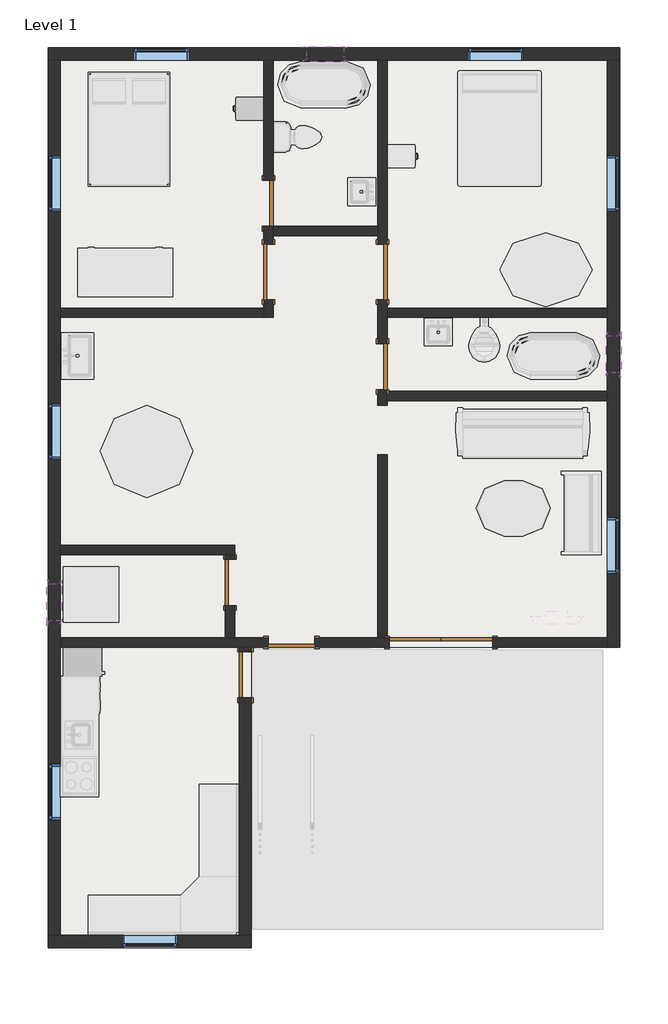
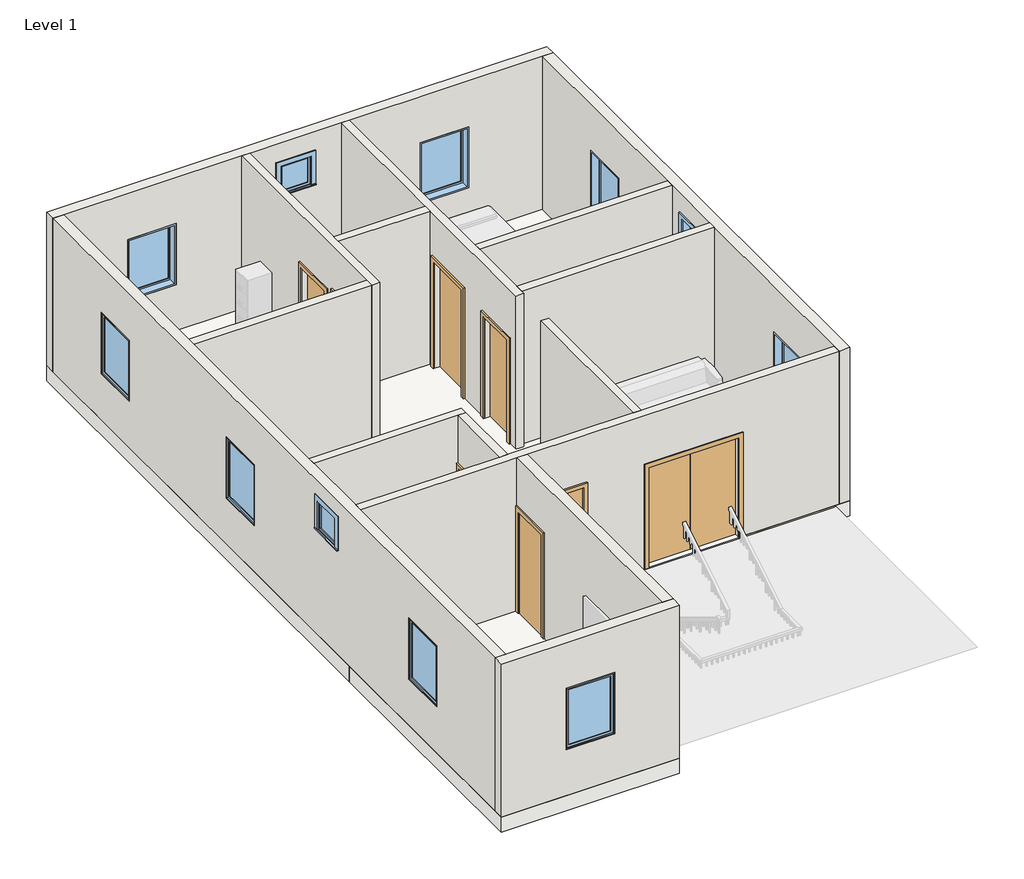
# One storey, part 1 of 3: 15 walls, 11 windows, 8 doors, 2 slabs.
"""IFC4 building model written with IfcOpenShell, lengths in millimetres."""

from ifc_helpers import new_model, si_unit, frame, origin, origin_with_axes, place, context, project, spatial, polyline, outline, extrude, faceted_brep, transform, mapped, element, save
from components import m_door_double_flush_panel_1700_x_2000mm_b668bbd0, door_059fdd7e, door_fadea3f2, door_686f89d2, door_16372e1c, window_e2841890, window_e41d21a6

model = new_model("IFC4")

# Units and contexts
model_context = context("Model", 3, world=origin())
ifc_project = project(units=[si_unit("LENGTHUNIT", "METRE", prefix="MILLI")], contexts=[model_context])

# Site, building, storey
site = spatial("IfcSite", under=ifc_project)
building = spatial("IfcBuilding", under=site)
storey = spatial("IfcBuildingStorey", under=building, Name="Level 1", Elevation=0.0)

# Doors
placement = place(None, origin())
m_door_double_flush_panel_1700_x_2000mm_shape = m_door_double_flush_panel_1700_x_2000mm_b668bbd0(model_context)
element("IfcDoor", 1, ObjectType="M_Door-Double-Flush_Panel : 1700 x 2000mm", at=placement, inside=storey, context=model_context, shape_type="MappedRepresentation", body=[
    mapped(m_door_double_flush_panel_1700_x_2000mm_shape, transform((-6764.5499219, 1169.9226537, 0.0), x_axis=(1.0, 0.0, 0.0), y_axis=(0.0, 1.0, 0.0), z_axis=(0.0, 0.0, 1.0))),
])
door_shape = door_059fdd7e(model_context)
element("IfcDoor", 2, ObjectType="Single-Flush : 30\" x 80\"", at=placement, inside=storey, context=model_context, shape_type="MappedRepresentation", body=[
    mapped(door_shape, transform((-9609.3499219, 8408.9226537, 0.0), x_axis=(0.0, -1.0, 0.0), y_axis=(1.0, 0.0, 0.0), z_axis=(0.0, 0.0, 1.0))),
])
element("IfcDoor", 3, ObjectType="Single-Flush : 30\" x 80\"", at=placement, inside=storey, context=model_context, shape_type="MappedRepresentation", body=[
    mapped(door_shape, transform((-7729.7499219, 5716.5226537, 0.0), x_axis=(0.0, -1.0, 0.0), y_axis=(1.0, 0.0, 0.0), z_axis=(0.0, 0.0, 1.0))),
])
element("IfcDoor", 4, ObjectType="Single-Flush : 30\" x 80\"", at=placement, inside=storey, context=model_context, shape_type="MappedRepresentation", body=[
    mapped(door_shape, transform((-10244.3499219, 2160.5226537, 0.0), x_axis=(0.0, 1.0, 0.0), y_axis=(-1.0, 0.0, 0.0), z_axis=(0.0, 0.0, 1.0))),
])
element("IfcDoor", 5, ObjectType="Single-Flush : 30\" x 80\"", at=placement, inside=storey, context=model_context, shape_type="MappedRepresentation", body=[
    mapped(door_shape, transform((-9228.3499219, 1169.9226537, 0.0), x_axis=(-1.0, 0.0, 0.0), y_axis=(0.0, -1.0, 0.0), z_axis=(0.0, 0.0, 1.0))),
])
door_2_shape = door_fadea3f2(model_context)
element("IfcDoor", 6, ObjectType="Single-Flush : 30\" x 80\"", at=placement, inside=storey, context=model_context, shape_type="MappedRepresentation", body=[
    mapped(door_2_shape, transform((-9990.3499219, 636.5226537, 0.0), x_axis=(0.0, 1.0, 0.0), y_axis=(-1.0, 0.0, 0.0), z_axis=(0.0, 0.0, 1.0))),
])
door_3_shape = door_686f89d2(model_context)
element("IfcDoor", 7, ObjectType="Single-Flush : 36\" x 84\"", at=placement, inside=storey, context=model_context, shape_type="MappedRepresentation", body=[
    mapped(door_3_shape, transform((-9609.3499219, 7278.6226537, 0.0), x_axis=(0.0, -1.0, 0.0), y_axis=(1.0, 0.0, 0.0), z_axis=(0.0, 0.0, 1.0))),
])
door_4_shape = door_16372e1c(model_context)
element("IfcDoor", 8, ObjectType="Single-Flush : 36\" x 84\"", at=placement, inside=storey, context=model_context, shape_type="MappedRepresentation", body=[
    mapped(door_4_shape, transform((-7729.7499219, 7278.6226537, 0.0), x_axis=(0.0, -1.0, 0.0), y_axis=(1.0, 0.0, 0.0), z_axis=(0.0, 0.0, 1.0))),
])

# Slabs
element("IfcSlab", 9, ObjectType="Generic - 12\"", at=placement, inside=storey, context=model_context, shape_type="SweptSolid", body=[
    extrude(outline(polyline([(-3818.1499219, 10974.3226537), (-3818.1499219, 1093.7226537), (-13241.5499219, 1093.7226537), (-13241.5499219, 10974.3226537), (-3818.1499219, 10974.3226537)])), frame((0.0, 0.0, -304.8), z_axis=(0.0, 0.0, 1.0), x_axis=(1.0, 0.0, 0.0)), (0.0, 0.0, 1.0), 304.8),
])
element("IfcSlab", 10, ObjectType="Generic - 12\"", at=placement, inside=storey, context=model_context, shape_type="SweptSolid", body=[
    extrude(outline(polyline([(-9888.7499219, 1093.7226537), (-9888.7499219, -3859.2773463), (-13241.5499219, -3859.2773463), (-13241.5499219, 1093.7226537), (-9888.7499219, 1093.7226537)])), frame((0.0, 0.0, -304.8), z_axis=(0.0, 0.0, 1.0), x_axis=(1.0, 0.0, 0.0)), (0.0, 0.0, 1.0), 304.8),
])

# Walls
element("IfcWall", 11, ObjectType="Generic - 8\"", at=placement, inside=storey, context=model_context, shape_type="Brep", body=[
    faceted_brep([(-13241.5499219, 10771.1226537, 0.0), (-13038.3499219, 10771.1226537, 0.0), (-9685.5499219, 10771.1226537, 0.0), (-9533.1499219, 10771.1226537, 0.0), (-7805.9499219, 10771.1226537, 0.0), (-7653.5499219, 10771.1226537, 0.0), (-4021.3499219, 10771.1226537, 0.0), (-3818.1499219, 10771.1226537, 0.0), (-3818.1499219, 10771.1226537, 3048.0), (-4021.3499219, 10771.1226537, 3048.0), (-7653.5499219, 10771.1226537, 3048.0), (-7805.9499219, 10771.1226537, 3048.0), (-9533.1499219, 10771.1226537, 3048.0), (-9685.5499219, 10771.1226537, 3048.0), (-13038.3499219, 10771.1226537, 3048.0), (-13241.5499219, 10771.1226537, 3048.0), (-10917.4499219, 10771.1226537, 2133.6), (-10917.4499219, 10771.1226537, 914.4), (-11831.8499219, 10771.1226537, 914.4), (-11831.8499219, 10771.1226537, 2133.6), (-5405.6499219, 10771.1226537, 2133.6), (-5405.6499219, 10771.1226537, 914.4), (-6320.0499219, 10771.1226537, 914.4), (-6320.0499219, 10771.1226537, 2133.6), (-8974.3499219, 10771.1226537, 2616.2), (-8364.7499219, 10771.1226537, 2616.2), (-8364.7499219, 10771.1226537, 2006.6), (-8974.3499219, 10771.1226537, 2006.6), (-13241.5499219, 10974.3226537, 0.0), (-13241.5499219, 10974.3226537, 3048.0), (-3818.1499219, 10974.3226537, 3048.0), (-3818.1499219, 10974.3226537, 0.0), (-10917.4499219, 10974.3226537, 2133.6), (-11831.8499219, 10974.3226537, 2133.6), (-11831.8499219, 10974.3226537, 914.4), (-10917.4499219, 10974.3226537, 914.4), (-5405.6499219, 10974.3226537, 2133.6), (-6320.0499219, 10974.3226537, 2133.6), (-6320.0499219, 10974.3226537, 914.4), (-5405.6499219, 10974.3226537, 914.4), (-8974.3499219, 10974.3226537, 2616.2), (-8974.3499219, 10974.3226537, 2006.6), (-8364.7499219, 10974.3226537, 2006.6), (-8364.7499219, 10974.3226537, 2616.2)], [[[0, 1, 2, 3, 4, 5, 6, 7, 8, 9, 10, 11, 12, 13, 14, 15], [16, 17, 18, 19], [20, 21, 22, 23], [24, 25, 26, 27]], [[28, 29, 30, 31], [32, 33, 34, 35], [36, 37, 38, 39], [40, 41, 42, 43]], [[7, 6, 5, 4, 3, 2, 1, 0, 28, 31]], [[15, 14, 13, 12, 11, 10, 9, 8, 30, 29]], [[8, 7, 31, 30]], [[0, 15, 29, 28]], [[17, 16, 32, 35]], [[18, 17, 35, 34]], [[19, 18, 34, 33]], [[16, 19, 33, 32]], [[21, 20, 36, 39]], [[22, 21, 39, 38]], [[23, 22, 38, 37]], [[20, 23, 37, 36]], [[41, 40, 24, 27]], [[42, 41, 27, 26]], [[43, 42, 26, 25]], [[40, 43, 25, 24]]]),
])
element("IfcWall", 12, ObjectType="Generic - 8\"", at=placement, inside=storey, context=model_context, shape_type="Brep", body=[
    faceted_brep([(-4021.3499219, 10771.1226537, 0.0), (-4021.3499219, 6681.7226537, 0.0), (-4021.3499219, 6529.3226537, 0.0), (-4021.3499219, 5310.1226537, 0.0), (-4021.3499219, 5157.7226537, 0.0), (-4021.3499219, 1246.1226537, 0.0), (-4021.3499219, 1093.7226537, 0.0), (-4021.3499219, 1093.7226537, 3048.0), (-4021.3499219, 1246.1226537, 3048.0), (-4021.3499219, 5157.7226537, 3048.0), (-4021.3499219, 5310.1226537, 3048.0), (-4021.3499219, 6529.3226537, 3048.0), (-4021.3499219, 6681.7226537, 3048.0), (-4021.3499219, 10771.1226537, 3048.0), (-4021.3499219, 8281.9226537, 2133.6), (-4021.3499219, 8281.9226537, 914.4), (-4021.3499219, 9196.3226537, 914.4), (-4021.3499219, 9196.3226537, 2133.6), (-4021.3499219, 2312.9226537, 2133.6), (-4021.3499219, 2312.9226537, 914.4), (-4021.3499219, 3227.3226537, 914.4), (-4021.3499219, 3227.3226537, 2133.6), (-4021.3499219, 5614.9226537, 2616.2), (-4021.3499219, 5614.9226537, 2006.6), (-4021.3499219, 6224.5226537, 2006.6), (-4021.3499219, 6224.5226537, 2616.2), (-3818.1499219, 10771.1226537, 0.0), (-3818.1499219, 10771.1226537, 3048.0), (-3818.1499219, 1093.7226537, 3048.0), (-3818.1499219, 1093.7226537, 0.0), (-3818.1499219, 8281.9226537, 2133.6), (-3818.1499219, 9196.3226537, 2133.6), (-3818.1499219, 9196.3226537, 914.4), (-3818.1499219, 8281.9226537, 914.4), (-3818.1499219, 2312.9226537, 2133.6), (-3818.1499219, 3227.3226537, 2133.6), (-3818.1499219, 3227.3226537, 914.4), (-3818.1499219, 2312.9226537, 914.4), (-3818.1499219, 5614.9226537, 2616.2), (-3818.1499219, 6224.5226537, 2616.2), (-3818.1499219, 6224.5226537, 2006.6), (-3818.1499219, 5614.9226537, 2006.6)], [[[0, 1, 2, 3, 4, 5, 6, 7, 8, 9, 10, 11, 12, 13], [14, 15, 16, 17], [18, 19, 20, 21], [22, 23, 24, 25]], [[26, 27, 28, 29], [30, 31, 32, 33], [34, 35, 36, 37], [38, 39, 40, 41]], [[6, 5, 4, 3, 2, 1, 0, 26, 29]], [[13, 12, 11, 10, 9, 8, 7, 28, 27]], [[0, 13, 27, 26]], [[7, 6, 29, 28]], [[15, 14, 30, 33]], [[16, 15, 33, 32]], [[17, 16, 32, 31]], [[14, 17, 31, 30]], [[19, 18, 34, 37]], [[20, 19, 37, 36]], [[21, 20, 36, 35]], [[18, 21, 35, 34]], [[23, 22, 38, 41]], [[24, 23, 41, 40]], [[25, 24, 40, 39]], [[22, 25, 39, 38]]]),
])
element("IfcWall", 13, ObjectType="Generic - 8\"", at=placement, inside=storey, context=model_context, shape_type="Brep", body=[
    faceted_brep([(-13038.3499219, -3656.0773463, 0.0), (-13038.3499219, 1093.7226537, 0.0), (-13038.3499219, 1246.1226537, 0.0), (-13038.3499219, 2617.7226537, 0.0), (-13038.3499219, 2770.1226537, 0.0), (-13038.3499219, 6529.3226537, 0.0), (-13038.3499219, 6681.7226537, 0.0), (-13038.3499219, 10771.1226537, 0.0), (-13038.3499219, 10771.1226537, 3048.0), (-13038.3499219, 6681.7226537, 3048.0), (-13038.3499219, 6529.3226537, 3048.0), (-13038.3499219, 2770.1226537, 3048.0), (-13038.3499219, 2617.7226537, 3048.0), (-13038.3499219, 1246.1226537, 3048.0), (-13038.3499219, 1093.7226537, 3048.0), (-13038.3499219, -3656.0773463, 3048.0), (-13038.3499219, -836.6773463, 2133.6), (-13038.3499219, -836.6773463, 914.4), (-13038.3499219, -1751.0773463, 914.4), (-13038.3499219, -1751.0773463, 2133.6), (-13038.3499219, 5106.9226537, 2133.6), (-13038.3499219, 5106.9226537, 914.4), (-13038.3499219, 4192.5226537, 914.4), (-13038.3499219, 4192.5226537, 2133.6), (-13038.3499219, 9196.3226537, 2133.6), (-13038.3499219, 9196.3226537, 914.4), (-13038.3499219, 8281.9226537, 914.4), (-13038.3499219, 8281.9226537, 2133.6), (-13038.3499219, 2135.1226537, 2692.4), (-13038.3499219, 2135.1226537, 2082.8), (-13038.3499219, 1525.5226537, 2082.8), (-13038.3499219, 1525.5226537, 2692.4), (-13241.5499219, -3656.0773463, 0.0), (-13241.5499219, -3656.0773463, 3048.0), (-13241.5499219, 10771.1226537, 3048.0), (-13241.5499219, 10771.1226537, 0.0), (-13241.5499219, -836.6773463, 2133.6), (-13241.5499219, -1751.0773463, 2133.6), (-13241.5499219, -1751.0773463, 914.4), (-13241.5499219, -836.6773463, 914.4), (-13241.5499219, 5106.9226537, 2133.6), (-13241.5499219, 4192.5226537, 2133.6), (-13241.5499219, 4192.5226537, 914.4), (-13241.5499219, 5106.9226537, 914.4), (-13241.5499219, 9196.3226537, 2133.6), (-13241.5499219, 8281.9226537, 2133.6), (-13241.5499219, 8281.9226537, 914.4), (-13241.5499219, 9196.3226537, 914.4), (-13241.5499219, 2135.1226537, 2692.4), (-13241.5499219, 1525.5226537, 2692.4), (-13241.5499219, 1525.5226537, 2082.8), (-13241.5499219, 2135.1226537, 2082.8)], [[[0, 1, 2, 3, 4, 5, 6, 7, 8, 9, 10, 11, 12, 13, 14, 15], [16, 17, 18, 19], [20, 21, 22, 23], [24, 25, 26, 27], [28, 29, 30, 31]], [[32, 33, 34, 35], [36, 37, 38, 39], [40, 41, 42, 43], [44, 45, 46, 47], [48, 49, 50, 51]], [[7, 6, 5, 4, 3, 2, 1, 0, 32, 35]], [[15, 14, 13, 12, 11, 10, 9, 8, 34, 33]], [[8, 7, 35, 34]], [[0, 15, 33, 32]], [[17, 16, 36, 39]], [[18, 17, 39, 38]], [[19, 18, 38, 37]], [[16, 19, 37, 36]], [[21, 20, 40, 43]], [[22, 21, 43, 42]], [[23, 22, 42, 41]], [[20, 23, 41, 40]], [[25, 24, 44, 47]], [[26, 25, 47, 46]], [[27, 26, 46, 45]], [[24, 27, 45, 44]], [[29, 28, 48, 51]], [[30, 29, 51, 50]], [[31, 30, 50, 49]], [[28, 31, 49, 48]]]),
])
element("IfcWall", 14, ObjectType="Generic - 8\"", at=placement, inside=storey, context=model_context, shape_type="SweptSolid", body=[
    extrude(outline(polyline([(1093.7226537, 0.0), (1017.5226537, 0.0), (1017.5226537, 2032.0), (255.5226537, 2032.0), (255.5226537, 0.0), (-3656.0773463, 0.0), (-3656.0773463, 3048.0), (1093.7226537, 3048.0), (1093.7226537, 0.0)])), frame((-10091.9499219, 0.0, 0.0), z_axis=(1.0, 0.0, 0.0), x_axis=(0.0, 1.0, 0.0)), (0.0, 0.0, 1.0), 203.2),
])
element("IfcWall", 15, ObjectType="Generic - 8\"", at=placement, inside=storey, context=model_context, shape_type="Brep", body=[
    faceted_brep([(-9888.7499219, -3656.0773463, 0.0), (-10091.9499219, -3656.0773463, 0.0), (-13038.3499219, -3656.0773463, 0.0), (-13241.5499219, -3656.0773463, 0.0), (-13241.5499219, -3656.0773463, 3048.0), (-13038.3499219, -3656.0773463, 3048.0), (-10091.9499219, -3656.0773463, 3048.0), (-9888.7499219, -3656.0773463, 3048.0), (-12022.3499219, -3656.0773463, 2133.6), (-12022.3499219, -3656.0773463, 914.4), (-11107.9499219, -3656.0773463, 914.4), (-11107.9499219, -3656.0773463, 2133.6), (-9888.7499219, -3859.2773463, 0.0), (-9888.7499219, -3859.2773463, 3048.0), (-13241.5499219, -3859.2773463, 3048.0), (-13241.5499219, -3859.2773463, 0.0), (-12022.3499219, -3859.2773463, 2133.6), (-11107.9499219, -3859.2773463, 2133.6), (-11107.9499219, -3859.2773463, 914.4), (-12022.3499219, -3859.2773463, 914.4)], [[[0, 1, 2, 3, 4, 5, 6, 7], [8, 9, 10, 11]], [[12, 13, 14, 15], [16, 17, 18, 19]], [[3, 2, 1, 0, 12, 15]], [[7, 6, 5, 4, 14, 13]], [[4, 3, 15, 14]], [[0, 7, 13, 12]], [[9, 8, 16, 19]], [[10, 9, 19, 18]], [[11, 10, 18, 17]], [[8, 11, 17, 16]]]),
])
element("IfcWall", 16, ObjectType="INNER WALL 6\"", at=placement, inside=storey, context=model_context, shape_type="Brep", body=[
    faceted_brep([(-9685.5499219, 8027.9226537, 2032.0), (-9685.5499219, 8027.9226537, 0.0), (-9685.5499219, 7735.8226537, 0.0), (-9685.5499219, 7735.8226537, 2133.6), (-9685.5499219, 6821.4226537, 2133.6), (-9685.5499219, 6821.4226537, 0.0), (-9685.5499219, 6681.7226537, 0.0), (-9685.5499219, 6529.3226537, 0.0), (-9685.5499219, 6529.3226537, 3048.0), (-9685.5499219, 6681.7226537, 3048.0), (-9685.5499219, 10771.1226537, 3048.0), (-9685.5499219, 10771.1226537, 0.0), (-9685.5499219, 8789.9226537, 0.0), (-9685.5499219, 8789.9226537, 2032.0), (-9533.1499219, 7735.8226537, 0.0), (-9533.1499219, 7875.5226537, 0.0), (-9533.1499219, 8027.9226537, 0.0), (-9533.1499219, 8027.9226537, 2032.0), (-9533.1499219, 8789.9226537, 2032.0), (-9533.1499219, 8789.9226537, 0.0), (-9533.1499219, 10771.1226537, 0.0), (-9533.1499219, 10771.1226537, 3048.0), (-9533.1499219, 8027.9226537, 3048.0), (-9533.1499219, 7875.5226537, 3048.0), (-9533.1499219, 6529.3226537, 3048.0), (-9533.1499219, 6529.3226537, 0.0), (-9533.1499219, 6821.4226537, 0.0), (-9533.1499219, 6821.4226537, 2133.6), (-9533.1499219, 7735.8226537, 2133.6)], [[[0, 1, 2, 3, 4, 5, 6, 7, 8, 9, 10, 11, 12, 13]], [[14, 15, 16, 17, 18, 19, 20, 21, 22, 23, 24, 25, 26, 27, 28]], [[7, 6, 5, 26, 25]], [[12, 11, 20, 19]], [[2, 1, 16, 15, 14]], [[10, 9, 8, 24, 23, 22, 21]], [[11, 10, 21, 20]], [[8, 7, 25, 24]], [[27, 26, 5, 4]], [[28, 27, 4, 3]], [[14, 28, 3, 2]], [[17, 16, 1, 0]], [[18, 17, 0, 13]], [[19, 18, 13, 12]]]),
])
element("IfcWall", 17, ObjectType="INNER WALL 6\"", at=placement, inside=storey, context=model_context, shape_type="SweptSolid", body=[
    extrude(outline(polyline([(-13038.3499219, 6681.7226537), (-9685.5499219, 6681.7226537), (-9685.5499219, 6529.3226537), (-13038.3499219, 6529.3226537), (-13038.3499219, 6681.7226537)])), origin_with_axes(), (0.0, 0.0, 1.0), 3048.0),
])
element("IfcWall", 18, ObjectType="INNER WALL 6\"", at=placement, inside=storey, context=model_context, shape_type="Brep", body=[
    faceted_brep([(-7805.9499219, 8027.9226537, 0.0), (-9533.1499219, 8027.9226537, 0.0), (-9533.1499219, 8027.9226537, 2032.0), (-9533.1499219, 8027.9226537, 3048.0), (-7805.9499219, 8027.9226537, 3048.0), (-7805.9499219, 7875.5226537, 0.0), (-7805.9499219, 7875.5226537, 3048.0), (-9533.1499219, 7875.5226537, 3048.0), (-9533.1499219, 7875.5226537, 0.0)], [[[0, 1, 2, 3, 4]], [[5, 6, 7, 8]], [[1, 0, 5, 8]], [[4, 3, 7, 6]], [[0, 4, 6, 5]], [[3, 2, 1, 8, 7]]]),
])
element("IfcWall", 19, ObjectType="INNER WALL 6\"", at=placement, inside=storey, context=model_context, shape_type="SweptSolid", body=[
    extrude(outline(polyline([(-4021.3499219, 6529.3226537), (-7653.5499219, 6529.3226537), (-7653.5499219, 6681.7226537), (-4021.3499219, 6681.7226537), (-4021.3499219, 6529.3226537)])), origin_with_axes(), (0.0, 0.0, 1.0), 3048.0),
])
element("IfcWall", 20, ObjectType="INNER WALL 6\"", at=placement, inside=storey, context=model_context, shape_type="Brep", body=[
    faceted_brep([(-13038.3499219, 2617.7226537, 0.0), (-10320.5499219, 2617.7226537, 0.0), (-10168.1499219, 2617.7226537, 0.0), (-10168.1499219, 2617.7226537, 3048.0), (-10320.5499219, 2617.7226537, 3048.0), (-13038.3499219, 2617.7226537, 3048.0), (-13038.3499219, 2770.1226537, 0.0), (-13038.3499219, 2770.1226537, 3048.0), (-10168.1499219, 2770.1226537, 3048.0), (-10168.1499219, 2770.1226537, 0.0)], [[[0, 1, 2, 3, 4, 5]], [[6, 7, 8, 9]], [[2, 1, 0, 6, 9]], [[5, 4, 3, 8, 7]], [[0, 5, 7, 6]], [[3, 2, 9, 8]]]),
])
element("IfcWall", 21, ObjectType="INNER WALL 6\"", at=placement, inside=storey, context=model_context, shape_type="Brep", body=[
    faceted_brep([(-4021.3499219, 1093.7226537, 3048.0), (-9888.7499219, 1093.7226537, 3048.0), (-10091.9499219, 1093.7226537, 3048.0), (-13038.3499219, 1093.7226537, 3048.0), (-13038.3499219, 1093.7226537, 0.0), (-10091.9499219, 1093.7226537, 0.0), (-9888.7499219, 1093.7226537, 0.0), (-9609.3499219, 1093.7226537, 0.0), (-9609.3499219, 1093.7226537, 2032.0), (-8847.3499219, 1093.7226537, 2032.0), (-8847.3499219, 1093.7226537, 0.0), (-7614.5499219, 1093.7226537, 0.0), (-7614.5499219, 1093.7226537, 2000.0), (-5914.5499219, 1093.7226537, 2000.0), (-5914.5499219, 1093.7226537, 0.0), (-4021.3499219, 1093.7226537, 0.0), (-13038.3499219, 1246.1226537, 3048.0), (-10320.5499219, 1246.1226537, 3048.0), (-10168.1499219, 1246.1226537, 3048.0), (-7805.9499219, 1246.1226537, 3048.0), (-7653.5499219, 1246.1226537, 3048.0), (-4021.3499219, 1246.1226537, 3048.0), (-4021.3499219, 1246.1226537, 0.0), (-5914.5499219, 1246.1226537, 0.0), (-5914.5499219, 1246.1226537, 2000.0), (-7614.5499219, 1246.1226537, 2000.0), (-7614.5499219, 1246.1226537, 0.0), (-7653.5499219, 1246.1226537, 0.0), (-7805.9499219, 1246.1226537, 0.0), (-8847.3499219, 1246.1226537, 0.0), (-8847.3499219, 1246.1226537, 2032.0), (-9609.3499219, 1246.1226537, 2032.0), (-9609.3499219, 1246.1226537, 0.0), (-10168.1499219, 1246.1226537, 0.0), (-10320.5499219, 1246.1226537, 0.0), (-13038.3499219, 1246.1226537, 0.0)], [[[0, 1, 2, 3, 4, 5, 6, 7, 8, 9, 10, 11, 12, 13, 14, 15]], [[16, 17, 18, 19, 20, 21, 22, 23, 24, 25, 26, 27, 28, 29, 30, 31, 32, 33, 34, 35]], [[4, 35, 34, 33, 32, 7, 6, 5]], [[22, 15, 14, 23]], [[10, 29, 28, 27, 26, 11]], [[3, 2, 1, 0, 21, 20, 19, 18, 17, 16]], [[4, 3, 16, 35]], [[0, 15, 22, 21]], [[8, 7, 32, 31]], [[9, 8, 31, 30]], [[10, 9, 30, 29]], [[13, 24, 23, 14]], [[24, 13, 12, 25]], [[25, 12, 11, 26]]]),
])
element("IfcWall", 22, ObjectType="INNER WALL 6\"", at=placement, inside=storey, context=model_context, shape_type="SweptSolid", body=[
    extrude(outline(polyline([(-7653.5499219, 4268.7226537), (-7653.5499219, 1246.1226537), (-7805.9499219, 1246.1226537), (-7805.9499219, 4268.7226537), (-7653.5499219, 4268.7226537)])), origin_with_axes(), (0.0, 0.0, 1.0), 3048.0),
])
element("IfcWall", 23, ObjectType="INNER WALL 6\"", at=placement, inside=storey, context=model_context, shape_type="SweptSolid", body=[
    extrude(outline(polyline([(-4021.3499219, 5157.7226537), (-7653.5499219, 5157.7226537), (-7653.5499219, 5310.1226537), (-4021.3499219, 5310.1226537), (-4021.3499219, 5157.7226537)])), origin_with_axes(), (0.0, 0.0, 1.0), 3048.0),
])
element("IfcWall", 24, ObjectType="INNER WALL 6\"", at=placement, inside=storey, context=model_context, shape_type="SweptSolid", body=[
    extrude(outline(polyline([(2617.7226537, 0.0), (2541.5226537, 0.0), (2541.5226537, 2032.0), (1779.5226537, 2032.0), (1779.5226537, 0.0), (1246.1226537, 0.0), (1246.1226537, 3048.0), (2617.7226537, 3048.0), (2617.7226537, 0.0)])), frame((-10320.5499219, 0.0, 0.0), z_axis=(1.0, 0.0, 0.0), x_axis=(0.0, 1.0, 0.0)), (0.0, 0.0, 1.0), 152.4),
])
element("IfcWall", 25, ObjectType="INNER WALL 6\"", at=placement, inside=storey, context=model_context, shape_type="Brep", body=[
    faceted_brep([(-7653.5499219, 5081.5226537, 0.0), (-7653.5499219, 5157.7226537, 0.0), (-7653.5499219, 5310.1226537, 0.0), (-7653.5499219, 5335.5226537, 0.0), (-7653.5499219, 5335.5226537, 2032.0), (-7653.5499219, 6097.5226537, 2032.0), (-7653.5499219, 6097.5226537, 0.0), (-7653.5499219, 6529.3226537, 0.0), (-7653.5499219, 6681.7226537, 0.0), (-7653.5499219, 6821.4226537, 0.0), (-7653.5499219, 6821.4226537, 2133.6), (-7653.5499219, 7735.8226537, 2133.6), (-7653.5499219, 7735.8226537, 0.0), (-7653.5499219, 10771.1226537, 0.0), (-7653.5499219, 10771.1226537, 3048.0), (-7653.5499219, 6681.7226537, 3048.0), (-7653.5499219, 6529.3226537, 3048.0), (-7653.5499219, 5310.1226537, 3048.0), (-7653.5499219, 5157.7226537, 3048.0), (-7653.5499219, 5081.5226537, 3048.0), (-7805.9499219, 5335.5226537, 2032.0), (-7805.9499219, 5335.5226537, 0.0), (-7805.9499219, 5081.5226537, 0.0), (-7805.9499219, 5081.5226537, 3048.0), (-7805.9499219, 7875.5226537, 3048.0), (-7805.9499219, 8027.9226537, 3048.0), (-7805.9499219, 10771.1226537, 3048.0), (-7805.9499219, 10771.1226537, 0.0), (-7805.9499219, 8027.9226537, 0.0), (-7805.9499219, 7875.5226537, 0.0), (-7805.9499219, 7735.8226537, 0.0), (-7805.9499219, 7735.8226537, 2133.6), (-7805.9499219, 6821.4226537, 2133.6), (-7805.9499219, 6821.4226537, 0.0), (-7805.9499219, 6097.5226537, 0.0), (-7805.9499219, 6097.5226537, 2032.0)], [[[0, 1, 2, 3, 4, 5, 6, 7, 8, 9, 10, 11, 12, 13, 14, 15, 16, 17, 18, 19]], [[20, 21, 22, 23, 24, 25, 26, 27, 28, 29, 30, 31, 32, 33, 34, 35]], [[34, 33, 9, 8, 7, 6]], [[22, 21, 3, 2, 1, 0]], [[30, 29, 28, 27, 13, 12]], [[19, 18, 17, 16, 15, 14, 26, 25, 24, 23]], [[0, 19, 23, 22]], [[14, 13, 27, 26]], [[12, 11, 31, 30]], [[11, 10, 32, 31]], [[10, 9, 33, 32]], [[6, 5, 35, 34]], [[5, 4, 20, 35]], [[4, 3, 21, 20]]]),
])

# Windows
window_shape = window_e2841890(model_context)
element("IfcWindow", 26, ObjectType="Fixed : 36\" x 48\"", at=placement, inside=storey, context=model_context, shape_type="MappedRepresentation", body=[
    mapped(window_shape, transform((-11603.2499219, -3757.6773463, 0.0), x_axis=(-1.0, 0.0, 0.0), y_axis=(0.0, -1.0, 0.0), z_axis=(0.0, 0.0, 1.0))),
])
element("IfcWindow", 27, ObjectType="Fixed : 36\" x 48\"", at=placement, inside=storey, context=model_context, shape_type="MappedRepresentation", body=[
    mapped(window_shape, transform((-13139.9499219, -1255.7773463, 0.0), x_axis=(0.0, 1.0, 0.0), y_axis=(-1.0, 0.0, 0.0), z_axis=(0.0, 0.0, 1.0))),
])
element("IfcWindow", 28, ObjectType="Fixed : 36\" x 48\"", at=placement, inside=storey, context=model_context, shape_type="MappedRepresentation", body=[
    mapped(window_shape, transform((-13139.9499219, 4687.8226537, 0.0), x_axis=(0.0, 1.0, 0.0), y_axis=(-1.0, 0.0, 0.0), z_axis=(0.0, 0.0, 1.0))),
])
element("IfcWindow", 29, ObjectType="Fixed : 36\" x 48\"", at=placement, inside=storey, context=model_context, shape_type="MappedRepresentation", body=[
    mapped(window_shape, transform((-13139.9499219, 8777.2226537, 0.0), x_axis=(0.0, 1.0, 0.0), y_axis=(-1.0, 0.0, 0.0), z_axis=(0.0, 0.0, 1.0))),
])
element("IfcWindow", 30, ObjectType="Fixed : 36\" x 48\"", at=placement, inside=storey, context=model_context, shape_type="MappedRepresentation", body=[
    mapped(window_shape, transform((-11336.5499219, 10872.7226537, 0.0), x_axis=(1.0, 0.0, 0.0), y_axis=(0.0, 1.0, 0.0), z_axis=(0.0, 0.0, 1.0))),
])
element("IfcWindow", 31, ObjectType="Fixed : 36\" x 48\"", at=placement, inside=storey, context=model_context, shape_type="MappedRepresentation", body=[
    mapped(window_shape, transform((-5824.7499219, 10872.7226537, 0.0), x_axis=(1.0, 0.0, 0.0), y_axis=(0.0, 1.0, 0.0), z_axis=(0.0, 0.0, 1.0))),
])
element("IfcWindow", 32, ObjectType="Fixed : 36\" x 48\"", at=placement, inside=storey, context=model_context, shape_type="MappedRepresentation", body=[
    mapped(window_shape, transform((-3919.7499219, 8701.0226537, 0.0), x_axis=(0.0, -1.0, 0.0), y_axis=(1.0, 0.0, 0.0), z_axis=(0.0, 0.0, 1.0))),
])
element("IfcWindow", 33, ObjectType="Fixed : 36\" x 48\"", at=placement, inside=storey, context=model_context, shape_type="MappedRepresentation", body=[
    mapped(window_shape, transform((-3919.7499219, 2732.0226537, 0.0), x_axis=(0.0, -1.0, 0.0), y_axis=(1.0, 0.0, 0.0), z_axis=(0.0, 0.0, 1.0))),
])
window_2_shape = window_e41d21a6(model_context)
element("IfcWindow", 34, ObjectType="Transom with Trim : 24\" x 24\"", at=placement, inside=storey, context=model_context, shape_type="MappedRepresentation", body=[
    mapped(window_2_shape, transform((-13139.9499219, 1868.4226537, -76.2), x_axis=(0.0, 1.0, 0.0), y_axis=(-1.0, 0.0, 0.0), z_axis=(0.0, 0.0, 1.0))),
])
element("IfcWindow", 35, ObjectType="Transom with Trim : 24\" x 24\"", at=placement, inside=storey, context=model_context, shape_type="MappedRepresentation", body=[
    mapped(window_2_shape, transform((-8707.6499219, 10872.7226537, -152.4), x_axis=(-1.0, 0.0, 0.0), y_axis=(0.0, -1.0, 0.0), z_axis=(0.0, 0.0, 1.0))),
])
element("IfcWindow", 36, ObjectType="Transom with Trim : 24\" x 24\"", at=placement, inside=storey, context=model_context, shape_type="MappedRepresentation", body=[
    mapped(window_2_shape, transform((-3919.7499219, 5881.6226537, -152.4), x_axis=(0.0, -1.0, 0.0), y_axis=(1.0, 0.0, 0.0), z_axis=(0.0, 0.0, 1.0))),
])

save(model, "model.ifc")

# Revit data of these elements
# Type "M_Door-Double-Flush_Panel : 1700 x 2000mm"
#   Type Mark = "8"
#   Construction Type Id = "DOOR"
#   Assembly Code = "C1020"
#   Analytic Construction = "Wooden"
#   Thickness = 0' - 1.9685"
#   Thermal Resistance (R) = 2.5876 (h·ft²·°F)/BTU
#   Swing Angle [instance default] = 90.00°
#   Panel Width = 2' - 9.46457"
#   Heat Transfer Coefficient (U) = 0.3865 BTU/(h·ft²·°F)
#   Height = 6' - 6.74016"
#   Trim Projection Ext = 0' - 0.98425"
#   Trim Projection Int = 0' - 0.98425"
#   Trim Width = 0' - 3.14961"
#   Width = 5' - 6.92913"
#   Define Thermal Properties by = 1
#   Panel Material = Wood - Birch - Solid Stained Light Low Gloss
#   Trim Material = Paint - Sienna
#   Visual Light Transmittance = 0
#   Solar Heat Gain Coefficient = 0
#   Function = (empty or 0)
#   Wall Closure = (empty or 0)
# Type "Single-Flush : 30\" x 80\""
#   Type Mark = "5"
#   Construction Type Id = "MDOOR"
#   Assembly Code = "C1020"
#   Analytic Construction = "Metal"
#   Thickness = 0' - 2"
#   Heat Transfer Coefficient (U) = 0.651978 BTU/(h·ft²·°F)
#   Height = 6' - 8"
#   Trim Projection Ext = 0' - 1"
#   Trim Projection Int = 0' - 1"
#   Trim Width = 0' - 3"
#   Width = 2' - 6"
#   Define Thermal Properties by = 1
#   Door Material = Door - Panel
#   Frame Material = Door - Frame
#   Visual Light Transmittance = 0
#   Solar Heat Gain Coefficient = 0
#   Function = (empty or 0)
#   Wall Closure = (empty or 0)
# Type "Single-Flush : 36\" x 84\""
#   Type Mark = "1"
#   Construction Type Id = "MDOOR"
#   Assembly Code = "C1020"
#   Analytic Construction = "Metal"
#   Thickness = 0' - 2"
#   Heat Transfer Coefficient (U) = 0.651978 BTU/(h·ft²·°F)
#   Height = 7' - 0"
#   Trim Projection Ext = 0' - 1"
#   Trim Projection Int = 0' - 1"
#   Trim Width = 0' - 3"
#   Width = 3' - 0"
#   Define Thermal Properties by = 1
#   Door Material = Door - Panel
#   Frame Material = Door - Frame
#   Visual Light Transmittance = 0
#   Solar Heat Gain Coefficient = 0
#   Function = (empty or 0)
#   Wall Closure = (empty or 0)
# Type "Generic - 12\""
#   Assembly Code = "B1010"
#   Function = 0
#   Layers, outside or top first: 1' - 0" no material (function 1)
# Type "Generic - 8\""
#   Assembly Code = "B2010"
#   Layers, outside or top first: 0' - 8" no material (function 1)
# Type "INNER WALL 6\""
#   Assembly Code = "B2010"
#   Layers, outside or top first: 0' - 6" no material (function 1)
# Type "Fixed : 36\" x 48\""
#   Type Mark = "1"
#   Construction Type Id = "GSP4R"
#   Assembly Code = "B2020100"
#   Analytic Construction = "1/8 in Pilkington single glazing"
#   Visual Light Transmittance = 0.9
#   Solar Heat Gain Coefficient = 0.78
#   Heat Transfer Coefficient (U) = 0.6496 BTU/(h·ft²·°F)
#   Height = 4' - 0"
#   Default Sill Height = 3' - 0"
#   Width = 3' - 0"
#   Window Inset = 0' - 0 3/4"
#   Define Thermal Properties by = 1
#   Glass Pane Material = Glass
#   Sash Material = Sash
#   Wall Closure = (empty or 0)
# Type "Transom with Trim : 24\" x 24\""
#   Type Mark = "10"
#   Construction Type Id = "GSP4R"
#   Assembly Code = "B2020100"
#   Analytic Construction = "1/8 in Pilkington single glazing"
#   Visual Light Transmittance = 0.9
#   Solar Heat Gain Coefficient = 0.78
#   Heat Transfer Coefficient (U) = 0.6496 BTU/(h·ft²·°F)
#   Height = 2' - 0"
#   Default Sill Height = 7' - 1"
#   Trim Projection - Ext. = 0' - 0 1/2"
#   Trim Projection - Int. = 0' - 0 3/4"
#   Trim Width - Exterior = 0' - 3 1/2"
#   Trim Width - Interior = 0' - 3 1/2"
#   Width = 2' - 0"
#   Window Inset = 0' - 0 3/4"
#   Define Thermal Properties by = 1
#   Glass Pane Material = Glass
#   Sash Material = Sash
#   Trim Exterior Material = Trim
#   Trim Interior Material = Trim
#   Wall Closure = (empty or 0)
# Element 1 (IfcDoor, "M_Door-Double-Flush_Panel : 1700 x 2000mm")
#   Swing Angle = 90.00°
#   Phase Created = New Construction
#   Materials on its faces: "Paint - Sienna", "Wood - Birch - Solid Stained Light Low Gloss"
# Elements 2, 3, 4, 5, 6 (IfcDoor, "Single-Flush : 30\" x 80\"")
#   Phase Created = New Construction
#   Materials on its faces: "Door - Frame", "Door - Panel"
# Elements 7, 8 (IfcDoor, "Single-Flush : 36\" x 84\"")
#   Phase Created = New Construction
#   Materials on its faces: "Door - Frame", "Door - Panel"
# Elements 9, 10 (IfcSlab, "Generic - 12\"")
#   Height Offset From Level = 0' - 0"
#   Phase Created = New Construction
#   Materials on its faces: "Default Floor"
# Elements 11, 12, 13, 14, 15 (IfcWall, "Generic - 8\"")
#   Top Offset = 0' - 0"
#   Base Offset = 0' - 0"
#   Unconnected Height = 10' - 0"
#   wall height = 10' - 0"
#   Phase Created = New Construction
#   Base Constraint = Level 1
#   Materials on its faces: "Default Wall"
# Elements 16, 17, 18, 19, 20, 21, 22, 23, 24, 25 (IfcWall, "INNER WALL 6\"")
#   Top Offset = 0' - 0"
#   Base Offset = 0' - 0"
#   Unconnected Height = 10' - 0"
#   wall height = 10' - 0"
#   Phase Created = New Construction
#   Base Constraint = Level 1
#   Materials on its faces: "Default Wall"
# Element 26 (IfcWindow, "Fixed : 36\" x 48\"")
#   Mark = "1"
#   Phase Created = New Construction
#   Materials on its faces: "Sash", "Glass"
# Element 27 (IfcWindow, "Fixed : 36\" x 48\"")
#   Mark = "2"
#   Phase Created = New Construction
#   Materials on its faces: "Sash", "Glass"
# Element 28 (IfcWindow, "Fixed : 36\" x 48\"")
#   Mark = "3"
#   Phase Created = New Construction
#   Materials on its faces: "Sash", "Glass"
# Element 29 (IfcWindow, "Fixed : 36\" x 48\"")
#   Mark = "4"
#   Phase Created = New Construction
#   Materials on its faces: "Sash", "Glass"
# Element 30 (IfcWindow, "Fixed : 36\" x 48\"")
#   Mark = "5"
#   Phase Created = New Construction
#   Materials on its faces: "Sash", "Glass"
# Element 31 (IfcWindow, "Fixed : 36\" x 48\"")
#   Mark = "6"
#   Phase Created = New Construction
#   Materials on its faces: "Sash", "Glass"
# Element 32 (IfcWindow, "Fixed : 36\" x 48\"")
#   Mark = "7"
#   Phase Created = New Construction
#   Materials on its faces: "Sash", "Glass"
# Element 33 (IfcWindow, "Fixed : 36\" x 48\"")
#   Mark = "8"
#   Phase Created = New Construction
#   Materials on its faces: "Sash", "Glass"
# Element 34 (IfcWindow, "Transom with Trim : 24\" x 24\"")
#   Mark = "9"
#   Phase Created = New Construction
#   Materials on its faces: "Sash", "Trim", "Glass"
# Element 35 (IfcWindow, "Transom with Trim : 24\" x 24\"")
#   Mark = "10"
#   Phase Created = New Construction
#   Materials on its faces: "Sash", "Trim", "Glass"
# Element 36 (IfcWindow, "Transom with Trim : 24\" x 24\"")
#   Mark = "11"
#   Phase Created = New Construction
#   Materials on its faces: "Sash", "Trim", "Glass"
# Materials
#   "Wood - Birch - Solid Stained Light Low Gloss": class "Wood", colour RGB 210 159 95, transparency 0, Cost = 0
#   "Paint - Sienna": colour RGB 118 70 51, transparency 0, Cost = 0
#   "Door - Panel": class "Wood", colour RGB 210 159 95, transparency 0
#   "Door - Frame": colour RGB 118 70 51, transparency 0
#   "Glass": class "Glass", colour RGB 0 128 192, transparency 0.75, Description = "Soda Lime Glass", Cost = 0
#   "Sash": class "Wood", colour RGB 224 178 126, transparency 0
#   "Trim": class "Wood", colour RGB 224 178 126, transparency 0
#   "Default Floor": colour RGB 128 128 128, transparency 0
#   "Default Wall": colour RGB 128 128 128, transparency 0
# Room at (-11252.715, 8461.513) mm, phase "New Construction", upper level "Level 1", upper offset 10' - 0", lower offset 0' - 0"
#   Number = "1"
#   Name = "BED ROOM 1"
# Room at (-8824.421, 9344.529) mm, phase "New Construction", upper level "Level 1", upper offset 10' - 0", lower offset 0' - 0"
#   Number = "2"
# Room at (-5561.085, 8461.513) mm, phase "New Construction", upper level "Level 1", upper offset 10' - 0", lower offset 0' - 0"
#   Number = "3"
#   Name = "BED ROOM 2"
# Room at (-10107.554, 4870.121) mm, phase "New Construction", upper level "Level 1", upper offset 10' - 0", lower offset 0' - 0"
#   Number = "4"
#   Name = "DINING HALL"
# Room at (-11659.29, 2014.117) mm, phase "New Construction", upper level "Level 1", upper offset 10' - 0", lower offset 0' - 0"
#   Number = "5"
# Room at (-11252.715, -207.22) mm, phase "New Construction", upper level "Level 1", upper offset 10' - 0", lower offset 0' - 0"
#   Number = "6"
#   Name = "KITCHEN"
# Room at (-5982.213, 2918.518) mm, phase "New Construction", upper level "Level 1", upper offset 10' - 0", lower offset 0' - 0"
#   Number = "7"
#   Name = "LIVING ROOM"
# Room at (-5982.213, 5726.923) mm, phase "New Construction", upper level "Level 1", upper offset 10' - 0", lower offset 0' - 0"
#   Number = "8"
